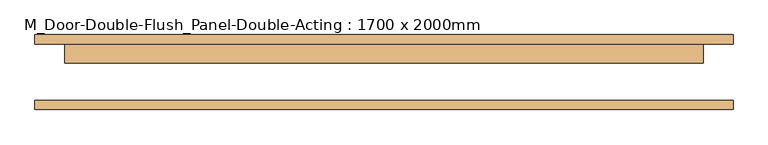
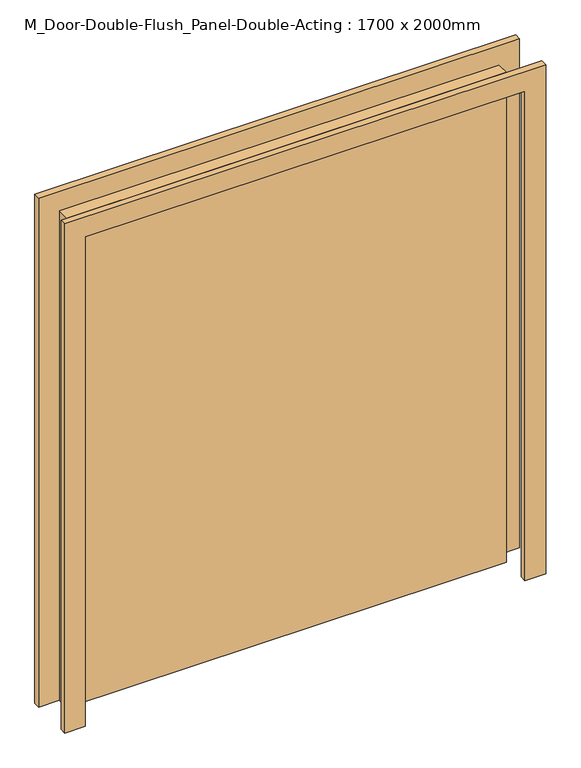
"""IFC4 building model written with IfcOpenShell, lengths in millimetres: door geometry, M_Door-Double-Flush_Panel-Double-Acting : 1700 x 2000mm."""

from ifc_helpers import new_model, si_unit, frame, origin, origin_with_axes, place, context, project, spatial, polyline, outline, extrude, source, transform, mapped, element, save


def m_door_double_flush_panel_double_acting_1700_x_2000mm_42eec5da(model_context):
    return source(origin(), model_context, "Body", "SweptSolid", [
        extrude(outline(polyline([(2080.0, -930.0), (0.0, -930.0), (0.0, -850.0), (2000.0, -850.0), (2000.0, 850.0), (0.0, 850.0), (0.0, 930.0), (2080.0, 930.0), (2080.0, -930.0)])), frame((0.0, 75.0, 0.0), z_axis=(0.0, 1.0, 0.0), x_axis=(0.0, 0.0, 1.0)), (0.0, 0.0, 1.0), 25.0),
        extrude(outline(polyline([(2000.0, -850.0), (2000.0, 850.0), (0.0, 850.0), (0.0, 930.0), (2080.0, 930.0), (2080.0, -930.0), (0.0, -930.0), (0.0, -850.0), (2000.0, -850.0)])), frame((0.0, -100.0, 0.0), z_axis=(0.0, 1.0, 0.0), x_axis=(0.0, 0.0, 1.0)), (0.0, 0.0, 1.0), 25.0),
        extrude(outline(polyline([(-850.0, 75.0), (850.0, 75.0), (850.0, 25.0), (-850.0, 25.0), (-850.0, 75.0)])), origin_with_axes(), (0.0, 0.0, 1.0), 2000.0),
    ])


if __name__ == "__main__":
    model = new_model("IFC4")
    model_context = context("Model", 3, world=origin())
    ifc_project = project(units=[si_unit("LENGTHUNIT", "METRE", prefix="MILLI")], contexts=[model_context])
    site = spatial("IfcSite", under=ifc_project)
    building = spatial("IfcBuilding", under=site)
    placement = place(None, origin())
    m_door_double_flush_panel_double_acting_1700_x_2000mm_shape = m_door_double_flush_panel_double_acting_1700_x_2000mm_42eec5da(model_context)
    element("IfcDoor", 1, ObjectType="M_Door-Double-Flush_Panel-Double-Acting : 1700 x 2000mm", at=placement, inside=building, context=model_context, shape_type="MappedRepresentation", body=[
        mapped(m_door_double_flush_panel_double_acting_1700_x_2000mm_shape, transform((0.0, 0.0, 0.0), x_axis=(1.0, 0.0, 0.0), y_axis=(0.0, 1.0, 0.0), z_axis=(0.0, 0.0, 1.0))),
    ])
    save(model, "model.ifc")

# Revit data of these elements
# Type "M_Door-Double-Flush_Panel-Double-Acting : 1700 x 2000mm"
#   Type Mark = "22"
#   Construction Type Id = "DOOR"
#   Assembly Code = "C1020"
#   Analytic Construction = "Wooden"
#   W = 850 mm
#   Thickness = 50 mm
#   Thermal Resistance (R) = 0.455703 (m²·K)/W
#   Swing Angle [instance default] = 90.00°
#   Heat Transfer Coefficient (U) = 2.19465 W/(m²·K)
#   Height = 2000 mm
#   Trim Projection Ext. = 25 mm
#   Trim Projection Int. = 25 mm
#   Trim Width Ext. = 80 mm
#   Trim Width Int. = 80 mm
#   Width = 1700 mm
#   Define Thermal Properties by = 1
#   Panel Material = Wood - Birch - Solid Stained Light Low Gloss
#   Trim Material = Paint - Sienna
#   Visual Light Transmittance = 0
#   Solar Heat Gain Coefficient = 0
#   Function = (empty or 0)
#   Wall Closure = (empty or 0)
# Element 1 (IfcDoor, "M_Door-Double-Flush_Panel-Double-Acting : 1700 x 2000mm")
#   Materials on its faces: "Paint - Sienna", "Wood - Birch - Solid Stained Light Low Gloss"
# Materials
#   "Wood - Birch - Solid Stained Light Low Gloss": class "Wood", colour RGB 210 159 95, transparency 0, Cost = 0
#   "Paint - Sienna": colour RGB 118 70 51, transparency 0, Cost = 0
